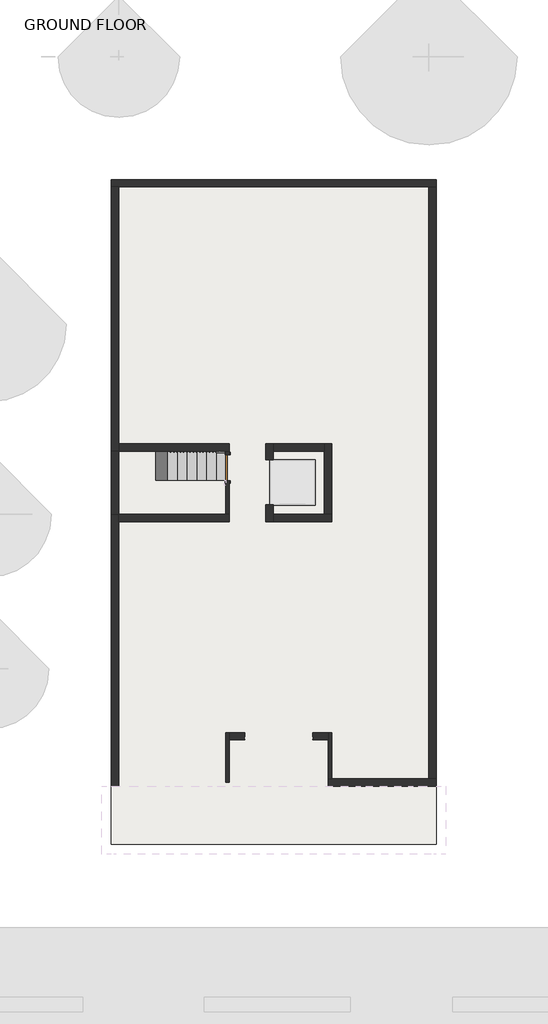
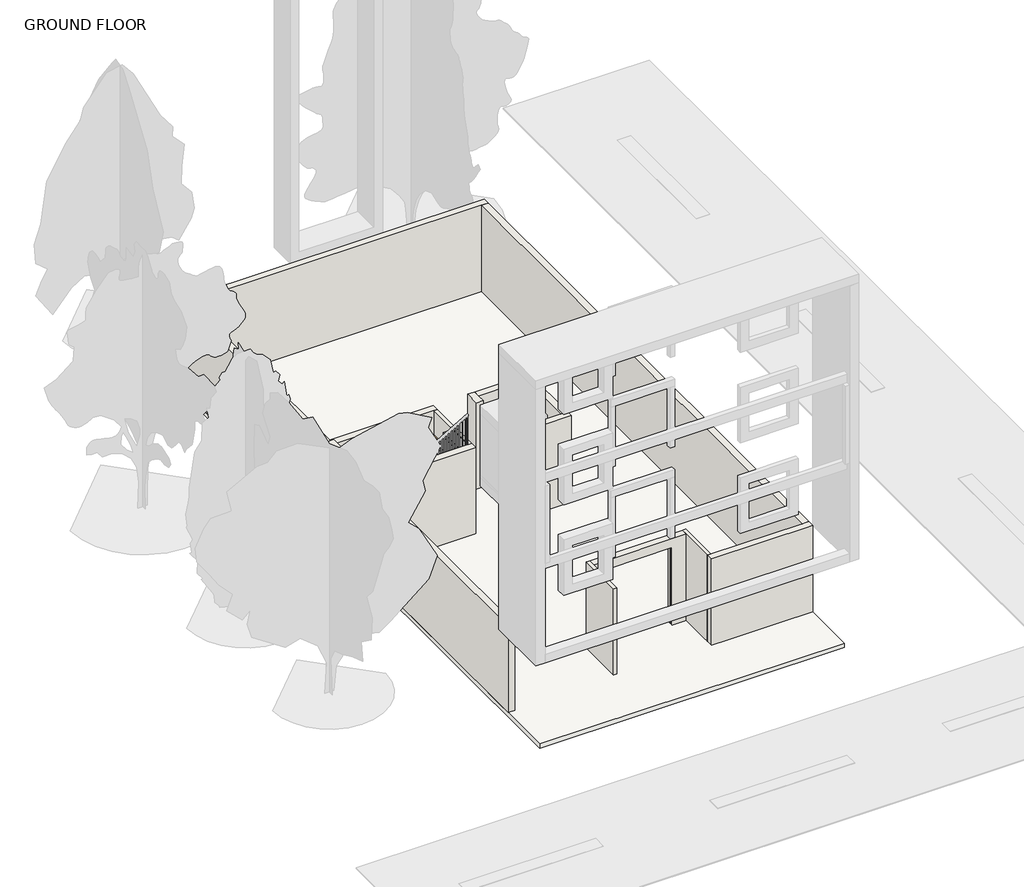
# One storey, part 1 of 2: 18 walls, 1 door, 1 slab, 1 stair flight.
"""IFC4 building model written with IfcOpenShell, lengths in millimetres."""

from ifc_helpers import new_model, si_unit, frame, origin, origin_with_axes, place, context, project, spatial, polyline, outline, extrude, faceted_brep, transform, mapped, element, save
from components import door_d141acb4

model = new_model("IFC4")

# Units and contexts
model_context = context("Model", 3, world=origin())
ifc_project = project(units=[si_unit("LENGTHUNIT", "METRE", prefix="MILLI")], contexts=[model_context])

# Site, building, storey
site = spatial("IfcSite", under=ifc_project)
building = spatial("IfcBuilding", under=site)
storey = spatial("IfcBuildingStorey", under=building, Name="GROUND FLOOR", Elevation=0.0)

# Door
placement = place(None, origin())
door_shape = door_d141acb4(model_context)
element("IfcDoor", 1, ObjectType="Single-Flush : 2'8\"X7'", at=placement, inside=storey, context=model_context, shape_type="MappedRepresentation", body=[
    mapped(door_shape, transform((-2719.6789041, 1029.1153263, 0.0), x_axis=(0.0, 1.0, 0.0), y_axis=(-1.0, 0.0, 0.0), z_axis=(0.0, 0.0, 1.0))),
])

# Slab
element("IfcSlab", 2, ObjectType="6\"", at=placement, inside=storey, context=model_context, shape_type="SweptSolid", body=[
    extrude(outline(polyline([(3814.4710959, 10058.8153263), (3814.4710959, -10769.1846737), (-6358.2289041, -10769.1846737), (-6358.2289041, 10058.8153263), (3814.4710959, 10058.8153263)])), frame((0.0, 0.0, -152.4), z_axis=(0.0, 0.0, 1.0), x_axis=(1.0, 0.0, 0.0)), (0.0, 0.0, 1.0), 152.4),
])

# Stair flight
element("IfcStairFlight", 3, ObjectType="3/4\" Nosing", at=placement, inside=storey, context=model_context, shape_type="Brep", body=[
    faceted_brep([(-2776.8289041, 635.4153263, 177.8), (-2776.8289041, 1549.8153263, 177.8), (-3100.6789041, 1549.8153263, 177.8), (-3100.6789041, 635.4153263, 177.8), (-3100.6789041, 635.4153263, 104.2858172), (-2921.9032174, 635.4153263, 0.0), (-2795.8789041, 635.4153263, 0.0), (-2795.8789041, 1549.8153263, 0.0), (-2921.9032174, 1549.8153263, 0.0), (-3100.6789041, 1549.8153263, 104.2858172), (-3081.6289041, 635.4153263, 355.6), (-3081.6289041, 1549.8153263, 355.6), (-3405.4789041, 1549.8153263, 355.6), (-3405.4789041, 635.4153263, 355.6), (-3405.4789041, 635.4153263, 282.0858172), (-3405.4789041, 1549.8153263, 282.0858172), (-3386.4289041, 635.4153263, 533.4), (-3386.4289041, 1549.8153263, 533.4), (-3710.2789041, 1549.8153263, 533.4), (-3710.2789041, 635.4153263, 533.4), (-3710.2789041, 635.4153263, 459.8858172), (-3710.2789041, 1549.8153263, 459.8858172), (-3691.2289041, 635.4153263, 711.2), (-3691.2289041, 1549.8153263, 711.2), (-4015.0789041, 1549.8153263, 711.2), (-4015.0789041, 635.4153263, 711.2), (-4015.0789041, 635.4153263, 637.6858172), (-4015.0789041, 1549.8153263, 637.6858172), (-3996.0289041, 635.4153263, 889.0), (-3996.0289041, 1549.8153263, 889.0), (-4319.8789041, 1549.8153263, 889.0), (-4319.8789041, 635.4153263, 889.0), (-4300.8289041, 635.4153263, 1066.8), (-4624.6789041, 635.4153263, 1066.8), (-4605.6289041, 635.4153263, 1244.6), (-4929.4789041, 635.4153263, 1244.6), (-4910.4289041, 635.4153263, 1422.4), (-5234.2789041, 635.4153263, 1422.4), (-5222.0324755, 635.4153263, 1536.7), (-5556.2460745, 635.4153263, 1536.7), (-4319.8789041, 1549.8153263, 815.4858172), (-4300.8289041, 1549.8153263, 1066.8), (-4624.6789041, 1549.8153263, 1066.8), (-4624.6789041, 1549.8153263, 993.2858172), (-4605.6289041, 1549.8153263, 1244.6), (-4929.4789041, 1549.8153263, 1244.6), (-4929.4789041, 1549.8153263, 1171.0858172), (-4910.4289041, 1549.8153263, 1422.4), (-5234.2789041, 1549.8153263, 1422.4), (-5234.2789041, 1549.8153263, 1348.8858172), (-5070.1545907, 483.0153263, 1600.2), (-2776.8289041, 483.0153263, 1600.2), (-2776.8289041, 635.4153263, 1600.2), (-3836.3032174, 635.4153263, 1600.2), (-5215.2289041, 635.4153263, 1600.2), (-5215.2289041, 1549.8153263, 1600.2), (-5556.2460745, 1549.8153263, 1600.2), (-6129.6289041, 1549.8153263, 1600.2), (-6129.6289041, -431.3846737, 1600.2), (-5196.1789041, -431.3846737, 1600.2), (-5196.1789041, 483.0153263, 1600.2), (-5179.0117336, 483.0153263, 1536.7), (-2776.8289041, 483.0153263, 1536.7), (-2776.8289041, 635.4153263, 1536.7), (-3727.4460745, 635.4153263, 1536.7), (-5556.2460745, 1549.8153263, 1536.7), (-6129.6289041, 1549.8153263, 1536.7), (-6129.6289041, -431.3846737, 1536.7), (-5196.1789041, -431.3846737, 1536.7), (-5215.2289041, 483.0153263, 1778.0), (-5215.2289041, -431.3846737, 1778.0), (-5179.0117336, -431.3846737, 1778.0), (-4891.3789041, -431.3846737, 1778.0), (-4891.3789041, 483.0153263, 1778.0), (-4891.3789041, 483.0153263, 1704.4858172), (-5179.0117336, -431.3846737, 1536.7), (-4891.3789041, -431.3846737, 1704.4858172), (-4910.4289041, 483.0153263, 1955.8), (-4910.4289041, -431.3846737, 1955.8), (-4586.5789041, -431.3846737, 1955.8), (-4586.5789041, 483.0153263, 1955.8), (-4586.5789041, 483.0153263, 1882.2858172), (-4586.5789041, -431.3846737, 1882.2858172), (-4605.6289041, 483.0153263, 2133.6), (-4605.6289041, -431.3846737, 2133.6), (-4281.7789041, -431.3846737, 2133.6), (-4281.7789041, 483.0153263, 2133.6), (-4281.7789041, 483.0153263, 2070.1), (-4281.7789041, 483.0153263, 2060.0858172), (-4598.8253326, 483.0153263, 2070.1), (-4281.7789041, -431.3846737, 2060.0858172), (-4300.8289041, 483.0153263, 2311.4), (-4300.8289041, -431.3846737, 2311.4), (-3976.9789041, -431.3846737, 2311.4), (-3976.9789041, 483.0153263, 2311.4), (-3976.9789041, 483.0153263, 2237.8858172), (-4264.6117336, 483.0153263, 2070.1), (-3976.9789041, -431.3846737, 2237.8858172), (-3996.0289041, 483.0153263, 2489.2), (-3996.0289041, -431.3846737, 2489.2), (-3672.1789041, -431.3846737, 2489.2), (-3672.1789041, 483.0153263, 2489.2), (-3672.1789041, 483.0153263, 2415.6858172), (-3672.1789041, -431.3846737, 2415.6858172), (-3691.2289041, 483.0153263, 2667.0), (-3691.2289041, -431.3846737, 2667.0), (-3367.3789041, -431.3846737, 2667.0), (-3367.3789041, 483.0153263, 2667.0), (-3367.3789041, 483.0153263, 2593.4858172), (-3367.3789041, -431.3846737, 2593.4858172), (-3386.4289041, 483.0153263, 2844.8), (-3386.4289041, -431.3846737, 2844.8), (-3062.5789041, -431.3846737, 2844.8), (-3062.5789041, 483.0153263, 2844.8), (-3062.5789041, 483.0153263, 2771.2858172), (-3062.5789041, -431.3846737, 2771.2858172), (-3081.6289041, 483.0153263, 3022.6), (-3081.6289041, -431.3846737, 3022.6), (-2776.8289041, -431.3846737, 3022.6), (-2776.8289041, 483.0153263, 3022.6), (-2776.8289041, 483.0153263, 2937.9733172), (-2776.8289041, -431.3846737, 2937.9733172)], [[[0, 1, 2, 3]], [[0, 3, 4, 5, 6]], [[2, 1, 7, 8, 9]], [[10, 11, 12, 13]], [[10, 13, 14, 4, 3]], [[12, 11, 2, 9, 15]], [[16, 17, 18, 19]], [[16, 19, 20, 14, 13]], [[18, 17, 12, 15, 21]], [[22, 23, 24, 25]], [[22, 25, 26, 20, 19]], [[24, 23, 18, 21, 27]], [[28, 29, 30, 31]], [[26, 25, 28, 31, 32, 33, 34, 35, 36, 37, 38, 39]], [[30, 29, 24, 27, 40]], [[32, 41, 42, 33]], [[42, 41, 30, 40, 43]], [[34, 44, 45, 35]], [[45, 44, 42, 43, 46]], [[36, 47, 48, 37]], [[48, 47, 45, 46, 49]], [[50, 51, 52, 53, 54, 55, 56, 57, 58, 59, 60]], [[50, 61, 62, 51]], [[52, 51, 62, 63]], [[52, 63, 64, 38, 54, 53]], [[55, 48, 49, 65, 66, 57, 56]], [[58, 57, 66, 67]], [[59, 58, 67, 68]], [[69, 70, 71, 72, 73]], [[69, 73, 74, 50, 60]], [[70, 59, 68, 75, 76, 72, 71]], [[77, 78, 79, 80]], [[77, 80, 81, 74, 73]], [[79, 78, 72, 76, 82]], [[83, 84, 85, 86]], [[83, 86, 87, 88, 81, 80, 89]], [[85, 84, 79, 82, 90]], [[91, 92, 93, 94]], [[91, 94, 95, 96, 88, 87, 86]], [[93, 92, 85, 90, 97]], [[98, 99, 100, 101]], [[98, 101, 102, 95, 94]], [[100, 99, 93, 97, 103]], [[104, 105, 106, 107]], [[104, 107, 108, 102, 101]], [[106, 105, 100, 103, 109]], [[110, 111, 112, 113]], [[110, 113, 114, 108, 107]], [[112, 111, 106, 109, 115]], [[1, 0, 6, 7]], [[3, 2, 11, 10]], [[13, 12, 17, 16]], [[19, 18, 23, 22]], [[25, 24, 29, 28]], [[31, 30, 41, 32]], [[33, 42, 44, 34]], [[35, 45, 47, 36]], [[37, 48, 55, 54, 38]], [[60, 59, 70, 69]], [[73, 72, 78, 77]], [[80, 79, 84, 83, 89]], [[86, 85, 92, 91]], [[94, 93, 99, 98]], [[101, 100, 105, 104]], [[107, 106, 111, 110]], [[116, 117, 118, 119]], [[116, 119, 120, 114, 113]], [[118, 117, 112, 115, 121]], [[119, 118, 121, 120]], [[113, 112, 117, 116]], [[7, 6, 5, 8]], [[26, 39, 65, 49, 46, 43, 40, 27, 21, 15, 9, 8, 5, 4, 14, 20]], [[65, 39, 38, 64, 63, 62, 61, 75, 68, 67, 66]], [[75, 61, 50, 74, 81, 88, 96, 95, 102, 108, 114, 120, 121, 115, 109, 103, 97, 90, 82, 76]]]),
])

# Walls
element("IfcWall", 4, ObjectType="4.5\"", at=placement, inside=storey, context=model_context, shape_type="SweptSolid", body=[
    extrude(outline(polyline([(1549.8153263, 0.0), (1435.5153263, 0.0), (1435.5153263, 2133.6), (622.7153263, 2133.6), (622.7153263, 0.0), (-431.3846737, 0.0), (-431.3846737, 3048.0), (1549.8153263, 3048.0), (1549.8153263, 0.0)])), frame((-2776.8289041, 0.0, 0.0), z_axis=(1.0, 0.0, 0.0), x_axis=(0.0, 1.0, 0.0)), (0.0, 0.0, 1.0), 114.3),
])
element("IfcWall", 5, ObjectType="4.5\"", at=placement, inside=storey, context=model_context, shape_type="Brep", body=[
    faceted_brep([(-2776.8289041, -7263.9846737, 0.0), (-2776.8289041, -8826.0846737, 0.0), (-2776.8289041, -8826.0846737, 3048.0), (-2776.8289041, -7263.9846737, 3048.0), (-2662.5289041, -7263.9846737, 0.0), (-2662.5289041, -7263.9846737, 3048.0), (-2662.5289041, -7492.5846737, 3048.0), (-2662.5289041, -8826.0846737, 3048.0), (-2662.5289041, -8826.0846737, 0.0), (-2662.5289041, -7492.5846737, 0.0)], [[[0, 1, 2, 3]], [[4, 5, 6, 7, 8, 9]], [[1, 0, 4, 9, 8]], [[2, 1, 8, 7]], [[3, 2, 7, 6, 5]], [[0, 3, 5, 4]]]),
])
element("IfcWall", 6, ObjectType="4.5\"", at=placement, inside=storey, context=model_context, shape_type="Brep", body=[
    faceted_brep([(537.8710959, -8711.7846737, 0.0), (537.8710959, -7263.9846737, 0.0), (537.8710959, -7263.9846737, 3048.0), (537.8710959, -8711.7846737, 3048.0), (423.5710959, -8711.7846737, 0.0), (423.5710959, -8711.7846737, 3048.0), (423.5710959, -7492.5846737, 3048.0), (423.5710959, -7263.9846737, 3048.0), (423.5710959, -7263.9846737, 0.0), (423.5710959, -7492.5846737, 0.0)], [[[0, 1, 2, 3]], [[4, 5, 6, 7, 8, 9]], [[1, 0, 4, 9, 8]], [[3, 2, 7, 6, 5]], [[0, 3, 5, 4]], [[2, 1, 8, 7]]]),
])
element("IfcWall", 7, ObjectType="9\"", at=placement, inside=storey, context=model_context, shape_type="Brep", body=[
    faceted_brep([(-1290.9289041, -659.9846737, 0.0), (537.8710959, -659.9846737, 0.0), (537.8710959, -659.9846737, 3048.0), (-1290.9289041, -659.9846737, 3048.0), (-1290.9289041, -431.3846737, 0.0), (-1290.9289041, -431.3846737, 3048.0), (309.2710959, -431.3846737, 3048.0), (537.8710959, -431.3846737, 3048.0), (537.8710959, -431.3846737, 0.0), (309.2710959, -431.3846737, 0.0)], [[[0, 1, 2, 3]], [[4, 5, 6, 7, 8, 9]], [[1, 0, 4, 9, 8]], [[3, 2, 7, 6, 5]], [[2, 1, 8, 7]], [[0, 3, 5, 4]]]),
])
element("IfcWall", 8, ObjectType="9\"", at=placement, inside=storey, context=model_context, shape_type="Brep", body=[
    faceted_brep([(537.8710959, -431.3846737, 0.0), (537.8710959, 1778.4153263, 0.0), (537.8710959, 1778.4153263, 3048.0), (537.8710959, -431.3846737, 3048.0), (309.2710959, -431.3846737, 0.0), (309.2710959, -431.3846737, 3048.0), (309.2710959, 1549.8153263, 3048.0), (309.2710959, 1778.4153263, 3048.0), (309.2710959, 1778.4153263, 0.0), (309.2710959, 1549.8153263, 0.0)], [[[0, 1, 2, 3]], [[4, 5, 6, 7, 8, 9]], [[1, 0, 4, 9, 8]], [[3, 2, 7, 6, 5]], [[0, 3, 5, 4]], [[2, 1, 8, 7]]]),
])
element("IfcWall", 9, ObjectType="9\"", at=placement, inside=storey, context=model_context, shape_type="Brep", body=[
    faceted_brep([(-2662.5289041, 1778.4153263, 0.0), (-6129.6289041, 1778.4153263, 0.0), (-6129.6289041, 1778.4153263, 3048.0), (-2662.5289041, 1778.4153263, 3048.0), (-2662.5289041, 1549.8153263, 0.0), (-2662.5289041, 1549.8153263, 3048.0), (-2776.8289041, 1549.8153263, 3048.0), (-6129.6289041, 1549.8153263, 3048.0), (-6129.6289041, 1549.8153263, 0.0), (-2776.8289041, 1549.8153263, 0.0)], [[[0, 1, 2, 3]], [[4, 5, 6, 7, 8, 9]], [[1, 0, 4, 9, 8]], [[3, 2, 7, 6, 5]], [[0, 3, 5, 4]], [[2, 1, 8, 7]]]),
])
element("IfcWall", 10, ObjectType="9\"", at=placement, inside=storey, context=model_context, shape_type="Brep", body=[
    faceted_brep([(-2662.5289041, -431.3846737, 0.0), (-2776.8289041, -431.3846737, 0.0), (-6129.6289041, -431.3846737, 0.0), (-6129.6289041, -431.3846737, 3048.0), (-2776.8289041, -431.3846737, 3048.0), (-2662.5289041, -431.3846737, 3048.0), (-2662.5289041, -659.9846737, 0.0), (-2662.5289041, -659.9846737, 3048.0), (-6129.6289041, -659.9846737, 3048.0), (-6129.6289041, -659.9846737, 0.0)], [[[0, 1, 2, 3, 4, 5]], [[6, 7, 8, 9]], [[2, 1, 0, 6, 9]], [[5, 4, 3, 8, 7]], [[0, 5, 7, 6]], [[3, 2, 9, 8]]]),
])
element("IfcWall", 11, ObjectType="9\"", at=placement, inside=storey, context=model_context, shape_type="SweptSolid", body=[
    extrude(outline(polyline([(-6358.2289041, -431.3846737), (-6358.2289041, 1549.8153263), (-6129.6289041, 1549.8153263), (-6129.6289041, -431.3846737), (-6358.2289041, -431.3846737)])), origin_with_axes(), (0.0, 0.0, 1.0), 3200.4),
])
element("IfcWall", 12, ObjectType="9\"", at=placement, inside=storey, context=model_context, shape_type="SweptSolid", body=[
    extrude(outline(polyline([(309.2710959, 1549.8153263), (-1290.9289041, 1549.8153263), (-1290.9289041, 1778.4153263), (309.2710959, 1778.4153263), (309.2710959, 1549.8153263)])), origin_with_axes(), (0.0, 0.0, 1.0), 3048.0),
])
element("IfcWall", 13, ObjectType="9\"", at=placement, inside=storey, context=model_context, shape_type="Brep", body=[
    faceted_brep([(-1519.5289041, 1778.4153263, 0.0), (-1519.5289041, 1273.6153263, 0.0), (-1519.5289041, 1273.6153263, 3048.0), (-1519.5289041, 1778.4153263, 3048.0), (-1290.9289041, 1778.4153263, 0.0), (-1290.9289041, 1778.4153263, 3048.0), (-1290.9289041, 1549.8153263, 3048.0), (-1290.9289041, 1273.6153263, 3048.0), (-1290.9289041, 1273.6153263, 0.0), (-1290.9289041, 1549.8153263, 0.0)], [[[0, 1, 2, 3]], [[4, 5, 6, 7, 8, 9]], [[1, 0, 4, 9, 8]], [[2, 1, 8, 7]], [[3, 2, 7, 6, 5]], [[0, 3, 5, 4]]]),
])
element("IfcWall", 14, ObjectType="9\"", at=placement, inside=storey, context=model_context, shape_type="Brep", body=[
    faceted_brep([(-1290.9289041, -659.9846737, 0.0), (-1290.9289041, -431.3846737, 0.0), (-1290.9289041, -126.3846737, 0.0), (-1290.9289041, -126.3846737, 3048.0), (-1290.9289041, -431.3846737, 3048.0), (-1290.9289041, -659.9846737, 3048.0), (-1519.5289041, -659.9846737, 0.0), (-1519.5289041, -659.9846737, 3048.0), (-1519.5289041, -126.3846737, 3048.0), (-1519.5289041, -126.3846737, 0.0)], [[[0, 1, 2, 3, 4, 5]], [[6, 7, 8, 9]], [[2, 1, 0, 6, 9]], [[3, 2, 9, 8]], [[5, 4, 3, 8, 7]], [[0, 5, 7, 6]]]),
])
element("IfcWall", 15, ObjectType="9\"", at=placement, inside=storey, context=model_context, shape_type="Brep", body=[
    faceted_brep([(-1519.5289041, 1778.4153263, 0.0), (-1519.5289041, 1273.6153263, 0.0), (-1519.5289041, 1273.6153263, 3048.0), (-1519.5289041, 1778.4153263, 3048.0), (-1290.9289041, 1778.4153263, 0.0), (-1290.9289041, 1778.4153263, 3048.0), (-1290.9289041, 1549.8153263, 3048.0), (-1290.9289041, 1273.6153263, 3048.0), (-1290.9289041, 1273.6153263, 0.0), (-1290.9289041, 1549.8153263, 0.0)], [[[0, 1, 2, 3]], [[4, 5, 6, 7, 8, 9]], [[1, 0, 4, 9, 8]], [[2, 1, 8, 7]], [[3, 2, 7, 6, 5]], [[0, 3, 5, 4]]]),
])
element("IfcWall", 16, ObjectType="9\"", at=placement, inside=storey, context=model_context, shape_type="Brep", body=[
    faceted_brep([(-1290.9289041, -659.9846737, 0.0), (-1290.9289041, -431.3846737, 0.0), (-1290.9289041, -126.3846737, 0.0), (-1290.9289041, -126.3846737, 3048.0), (-1290.9289041, -431.3846737, 3048.0), (-1290.9289041, -659.9846737, 3048.0), (-1519.5289041, -659.9846737, 0.0), (-1519.5289041, -659.9846737, 3048.0), (-1519.5289041, -126.3846737, 3048.0), (-1519.5289041, -126.3846737, 0.0)], [[[0, 1, 2, 3, 4, 5]], [[6, 7, 8, 9]], [[2, 1, 0, 6, 9]], [[3, 2, 9, 8]], [[5, 4, 3, 8, 7]], [[0, 5, 7, 6]]]),
])
element("IfcWall", 17, ObjectType="9\"", at=placement, inside=storey, context=model_context, shape_type="Brep", body=[
    faceted_brep([(423.5710959, -8940.3846737, 0.0), (3814.4710959, -8940.3846737, 0.0), (3814.4710959, -8940.3846737, 3048.0), (423.5710959, -8940.3846737, 3048.0), (423.5710959, -8711.7846737, 0.0), (423.5710959, -8711.7846737, 3048.0), (537.8710959, -8711.7846737, 3048.0), (3585.8710959, -8711.7846737, 3048.0), (3814.4710959, -8711.7846737, 3048.0), (3814.4710959, -8711.7846737, 0.0), (3585.8710959, -8711.7846737, 0.0), (537.8710959, -8711.7846737, 0.0)], [[[0, 1, 2, 3]], [[4, 5, 6, 7, 8, 9, 10, 11]], [[1, 0, 4, 11, 10, 9]], [[3, 2, 8, 7, 6, 5]], [[0, 3, 5, 4]], [[2, 1, 9, 8]]]),
])
element("IfcWall", 18, ObjectType="9\"", at=placement, inside=storey, context=model_context, shape_type="Brep", body=[
    faceted_brep([(423.5710959, -7492.5846737, 3048.0), (-2662.5289041, -7492.5846737, 3048.0), (-2662.5289041, -7492.5846737, 0.0), (-2186.2789041, -7492.5846737, 0.0), (-2186.2789041, -7492.5846737, 2743.2), (-52.6789041, -7492.5846737, 2743.2), (-52.6789041, -7492.5846737, 0.0), (423.5710959, -7492.5846737, 0.0), (-2662.5289041, -7263.9846737, 3048.0), (423.5710959, -7263.9846737, 3048.0), (423.5710959, -7263.9846737, 0.0), (-52.6789041, -7263.9846737, 0.0), (-52.6789041, -7263.9846737, 2743.2), (-2186.2789041, -7263.9846737, 2743.2), (-2186.2789041, -7263.9846737, 0.0), (-2662.5289041, -7263.9846737, 0.0), (-2186.2789041, -7402.5846737, 0.0), (-2201.2789041, -7402.5846737, 0.0), (-2201.2789041, -7472.5846737, 0.0), (-2186.2789041, -7472.5846737, 0.0), (-52.6789041, -7472.5846737, 0.0), (-37.6789041, -7472.5846737, 0.0), (-37.6789041, -7402.5846737, 0.0), (-52.6789041, -7402.5846737, 0.0), (-2186.2789041, -7472.5846737, 2743.2), (-52.6789041, -7472.5846737, 2743.2), (-52.6789041, -7402.5846737, 2743.2), (-2186.2789041, -7402.5846737, 2743.2), (-37.6789041, -7402.5846737, 2758.2), (-2201.2789041, -7402.5846737, 2758.2), (-2201.2789041, -7472.5846737, 2758.2), (-37.6789041, -7472.5846737, 2758.2)], [[[0, 1, 2, 3, 4, 5, 6, 7]], [[8, 9, 10, 11, 12, 13, 14, 15]], [[2, 15, 14, 16, 17, 18, 19, 3]], [[10, 7, 6, 20, 21, 22, 23, 11]], [[1, 0, 9, 8]], [[2, 1, 8, 15]], [[0, 7, 10, 9]], [[24, 25, 5, 4]], [[26, 27, 13, 12]], [[23, 26, 12, 11]], [[27, 16, 14, 13]], [[27, 26, 23, 22, 28, 29, 17, 16]], [[17, 29, 30, 18]], [[25, 24, 19, 18, 30, 31, 21, 20]], [[19, 24, 4, 3]], [[25, 20, 6, 5]], [[28, 22, 21, 31]], [[29, 28, 31, 30]]]),
])
element("IfcWall", 19, ObjectType="9\"", at=placement, inside=storey, context=model_context, shape_type="Brep", body=[
    faceted_brep([(3814.4710959, 10058.8153263, 0.0), (-6358.2289041, 10058.8153263, 0.0), (-6358.2289041, 10058.8153263, 3048.0), (3814.4710959, 10058.8153263, 3048.0), (3814.4710959, 9830.2153263, 0.0), (3814.4710959, 9830.2153263, 3048.0), (3585.8710959, 9830.2153263, 3048.0), (-6129.6289041, 9830.2153263, 3048.0), (-6358.2289041, 9830.2153263, 3048.0), (-6358.2289041, 9830.2153263, 0.0), (-6129.6289041, 9830.2153263, 0.0), (3585.8710959, 9830.2153263, 0.0)], [[[0, 1, 2, 3]], [[4, 5, 6, 7, 8, 9, 10, 11]], [[1, 0, 4, 11, 10, 9]], [[3, 2, 8, 7, 6, 5]], [[2, 1, 9, 8]], [[0, 3, 5, 4]]]),
])
element("IfcWall", 20, ObjectType="9\"", at=placement, inside=storey, context=model_context, shape_type="Brep", body=[
    faceted_brep([(-6358.2289041, 9830.2153263, 0.0), (-6358.2289041, -8940.3846737, 0.0), (-6358.2289041, -8940.3846737, 3048.0), (-6358.2289041, 9830.2153263, 3048.0), (-6129.6289041, 9830.2153263, 0.0), (-6129.6289041, 9830.2153263, 3048.0), (-6129.6289041, 1778.4153263, 3048.0), (-6129.6289041, 1549.8153263, 3048.0), (-6129.6289041, -431.3846737, 3048.0), (-6129.6289041, -659.9846737, 3048.0), (-6129.6289041, -8940.3846737, 3048.0), (-6129.6289041, -8940.3846737, 0.0), (-6129.6289041, -659.9846737, 0.0), (-6129.6289041, -431.3846737, 0.0), (-6129.6289041, 1549.8153263, 0.0), (-6129.6289041, 1778.4153263, 0.0)], [[[0, 1, 2, 3]], [[4, 5, 6, 7, 8, 9, 10, 11, 12, 13, 14, 15]], [[1, 0, 4, 15, 14, 13, 12, 11]], [[2, 1, 11, 10]], [[3, 2, 10, 9, 8, 7, 6, 5]], [[0, 3, 5, 4]]]),
])
element("IfcWall", 21, ObjectType="9\"", at=placement, inside=storey, context=model_context, shape_type="SweptSolid", body=[
    extrude(outline(polyline([(3585.8710959, -8711.7846737), (3585.8710959, 9830.2153263), (3814.4710959, 9830.2153263), (3814.4710959, -8711.7846737), (3585.8710959, -8711.7846737)])), origin_with_axes(), (0.0, 0.0, 1.0), 3048.0),
])

save(model, "model.ifc")

# Revit data of these elements
# Type "Single-Flush : 2'8\"X7'"
#   Type Mark = "12"
#   Construction Type Id = "MDOOR"
#   Assembly Code = "C1020"
#   Analytic Construction = "Metal"
#   Thickness = 0' - 2"
#   Heat Transfer Coefficient (U) = 0.651978 BTU/(h·ft²·°F)
#   Height = 7' - 0"
#   Trim Projection Ext = 0' - 1"
#   Trim Projection Int = 0' - 1"
#   Trim Width = 0' - 3"
#   Width = 2' - 8"
#   Define Thermal Properties by = 1
#   Door Material = Door - Panel
#   Frame Material = Door - Frame
#   Visual Light Transmittance = 0
#   Solar Heat Gain Coefficient = 0
#   Function = (empty or 0)
#   Wall Closure = (empty or 0)
# Type "6\""
#   Assembly Code = "B1010"
#   Function = 0
#   Layers, outside or top first: 0' - 6" no material (function 1)
# Type "4.5\""
#   Assembly Code = "B2010"
#   Layers, outside or top first: 0' - 4 1/2" no material (function 1)
# Type "9\""
#   Assembly Code = "B2010"
#   Layers, outside or top first: 0' - 9" "WALL" (function 1)
# Element 1 (IfcDoor, "Single-Flush : 2'8\"X7'")
#   Phase Created = New Construction
#   Materials on its faces: "Door - Frame", "Door - Panel"
# Element 2 (IfcSlab, "6\"")
#   Height Offset From Level = 0' - 0"
#   Phase Created = New Construction
#   Materials on its faces: "DUSTY ROSE", "Default Floor"
# Element 3 (IfcStairFlight, "3/4\" Nosing")
#   Phase Created = New Construction
#   Materials on its faces: "Concrete, Cast-in-Place gray"
# Element 4 (IfcWall, "4.5\"")
#   Top Offset = -0' - 6"
#   Base Offset = 0' - 0"
#   wall height = 10' - 0"
#   Phase Created = New Construction
#   Base Constraint = GROUND FLOOR
#   Top Constraint = FIRST FLOOR
#   Materials on its faces: "Default Wall"
# Elements 5, 6 (IfcWall, "4.5\"")
#   Top Offset = -0' - 6"
#   Base Offset = 0' - 0"
#   wall height = 10' - 0"
#   Phase Created = New Construction
#   Base Constraint = GROUND FLOOR
#   Top Constraint = FIRST FLOOR
#   Materials on its faces: "Default Wall", "WALL"
# Elements 7, 8, 12, 13, 14, 15, 16, 18 (IfcWall, "9\"")
#   Top Offset = -0' - 6"
#   Base Offset = 0' - 0"
#   wall height = 10' - 0"
#   Phase Created = New Construction
#   Base Constraint = GROUND FLOOR
#   Top Constraint = FIRST FLOOR
#   Materials on its faces: "WALL"
# Elements 9, 10 (IfcWall, "9\"")
#   Top Offset = -0' - 6"
#   Base Offset = 0' - 0"
#   wall height = 10' - 0"
#   Phase Created = New Construction
#   Base Constraint = GROUND FLOOR
#   Top Constraint = FIRST FLOOR
#   Materials on its faces: "WALL", "Default Wall"
# Element 11 (IfcWall, "9\"")
#   Top Offset = 0' - 0"
#   Base Offset = 0' - 0"
#   wall height = 10' - 6"
#   Phase Created = New Construction
#   Base Constraint = GROUND FLOOR
#   Top Constraint = FIRST FLOOR
#   Materials on its faces: "WALL", "6\" WALL"
# Element 17 (IfcWall, "9\"")
#   Top Offset = -0' - 6"
#   Base Offset = 0' - 0"
#   wall height = 10' - 0"
#   Phase Created = New Construction
#   Base Constraint = GROUND FLOOR
#   Top Constraint = FIRST FLOOR
#   Materials on its faces: "WALL", "Default Wall", "6\" WALL"
# Elements 19, 20, 21 (IfcWall, "9\"")
#   Top Offset = -0' - 6"
#   Base Offset = 0' - 0"
#   wall height = 10' - 0"
#   Phase Created = New Construction
#   Base Constraint = GROUND FLOOR
#   Top Constraint = FIRST FLOOR
#   Materials on its faces: "WALL", "6\" WALL"
# Materials
#   "Door - Panel": class "Wood", colour RGB 210 159 95, transparency 0, Cost = 0
#   "Door - Frame": colour RGB 118 70 51, transparency 0, Cost = 0
#   "WALL": class "Generic", colour RGB 84 102 113, transparency 0, Cost = 0
#   "DUSTY ROSE": class "Generic", colour RGB 120 120 120, transparency 0, Cost = 0
#   "Default Floor": colour RGB 128 128 128, transparency 0, Cost = 0
#   "Concrete, Cast-in-Place gray": class "Concrete", colour RGB 192 192 192, transparency 0, Description = "Cast-in-place concrete", Cost = 0
#   "Default Wall": colour RGB 128 128 128, transparency 0, Cost = 0
#   "6\" WALL": class "Generic", colour RGB 186 182 182, transparency 0, Cost = 0
